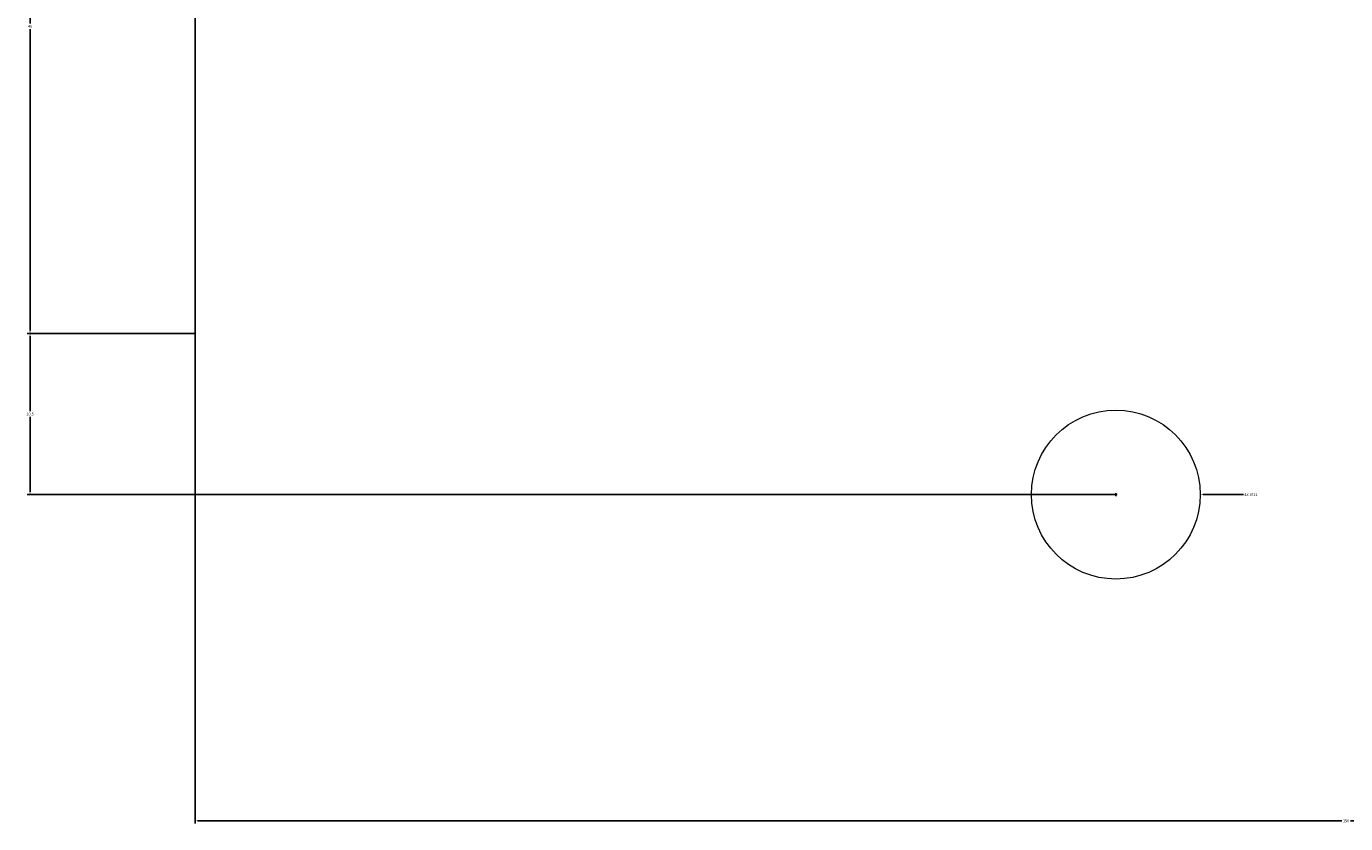
# Model space of a CAD drawing. Units: millimetres. Extents: x 315 to 487, y -72 to 32.
# Tile 1 of 4: x 315 to 401, y -72 to -20. Entities that reach past the tile are written whole.
import ezdxf

# ---------------------------------------------------------------- set-up
doc = ezdxf.new("R2010")
doc.units = ezdxf.units.MM
doc.layers.add('M-CONS', color=8, linetype='Continuous', lineweight=13)
doc.layers.add('M-DIMS', color=2, linetype='Continuous', lineweight=18)
doc.styles.get("Standard").update_dxf_attribs({"font": 'arial.ttf'})
doc.dimstyles.get("Standard").update_dxf_attribs({"dimtxt": 0.18, "dimasz": 0.18, "dimexe": 0.18, "dimexo": 0.0625, "dimgap": 0.09, "dimtad": 0, "dimtih": 1, "dimtoh": 1, "dimdec": 4, "dimzin": 0, "dimdsep": 46, "dimtxsty": 'Standard', "dimcen": 0.09, "dimadec": 0, "dimazin": 0, "dimtfac": 1, "dimtdec": 4, "dimtofl": 0, "dimtmove": 0, "dimatfit": 3, "dimfxl": 1, "dimtolj": 1, "dimtzin": 0, "dimarcsym": 0})

# ---------------------------------------------------------------- blocks, each defined once
blk = doc.blocks.new('*D3')
at = {"layer": 'Defpoints', "color": 0, "transparency": 16777216}
for p in [(326.007, 0), (476.007, 0), (476.007, -71.75)]:
    blk.add_point(p, dxfattribs=at)
at = {"layer": 'M-DIMS', "color": 0, "lineweight": -2, "transparency": 16777216}
for p, q in [((326.007, -0.062), (326.007, -71.93)), ((476.007, -0.062), (476.007, -71.93)), ((326.187, -71.75), (400.727, -71.75)), ((475.827, -71.75), (401.287, -71.75))]:
    blk.add_line(p, q, dxfattribs=at)
at = {"layer": 'M-DIMS', "color": 0, "transparency": 16777216}
for points in [[(326.187, -71.72), (326.187, -71.78), (326.007, -71.75)], [(475.827, -71.72), (475.827, -71.78), (476.007, -71.75)]]:
    blk.add_solid(points, dxfattribs=at)
at = {"layer": 'M-DIMS', "color": 0, "transparency": 16777216, "insert": (401.007, -71.75), "char_height": 0.18, "attachment_point": 5}
blk.add_mtext('\\A1;150', dxfattribs=at)
blk = doc.blocks.new('*D10')
at = {"layer": 'Defpoints', "color": 0, "transparency": 16777216}
for p in [(326.007, 0), (315.257, 0), (326.007, -40)]:
    blk.add_point(p, dxfattribs=at)
at = {"layer": 'M-DIMS', "color": 0, "lineweight": -2, "transparency": 16777216}
for p, q in [((325.945, 0), (315.077, 0)), ((315.257, -0.18), (315.257, -19.818)), ((315.257, -39.82), (315.257, -20.182)), ((325.945, -40), (315.077, -40))]:
    blk.add_line(p, q, dxfattribs=at)
at = {"layer": 'M-DIMS', "color": 0, "transparency": 16777216}
for points in [[(315.227, -0.18), (315.287, -0.18), (315.257, 0)], [(315.227, -39.82), (315.287, -39.82), (315.257, -40)]]:
    blk.add_solid(points, dxfattribs=at)
at = {"layer": 'M-DIMS', "color": 0, "transparency": 16777216, "insert": (315.257, -20), "char_height": 0.18, "attachment_point": 5}
blk.add_mtext('\\A1;40', dxfattribs=at)
blk = doc.blocks.new('*D13')
at = {"layer": 'Defpoints', "color": 0, "transparency": 16777216}
for p in [(315.257, -40), (326.007, -40), (386.007, -50.5)]:
    blk.add_point(p, dxfattribs=at)
at = {"layer": 'M-DIMS', "color": 0, "lineweight": -2, "transparency": 16777216}
for p, q in [((325.945, -40), (315.077, -40)), ((315.257, -40.18), (315.257, -45.068)), ((315.257, -50.32), (315.257, -45.432)), ((385.945, -50.5), (315.077, -50.5))]:
    blk.add_line(p, q, dxfattribs=at)
at = {"layer": 'M-DIMS', "color": 0, "transparency": 16777216}
for points in [[(315.227, -40.18), (315.287, -40.18), (315.257, -40)], [(315.227, -50.32), (315.287, -50.32), (315.257, -50.5)]]:
    blk.add_solid(points, dxfattribs=at)
at = {"layer": 'M-DIMS', "color": 0, "transparency": 16777216, "insert": (315.257, -45.25), "char_height": 0.18, "attachment_point": 5}
blk.add_mtext('\\A1;10.5', dxfattribs=at)
blk = doc.blocks.new('*D14')
at = {"layer": 'Defpoints', "color": 0, "transparency": 16777216}
for p in [(380.507, -50.5), (391.507, -50.5)]:
    blk.add_point(p, dxfattribs=at)
at = {"layer": 'M-DIMS', "color": 0, "lineweight": -2, "transparency": 16777216}
for p, q in [((385.917, -50.5), (386.097, -50.5)), ((386.007, -50.59), (386.007, -50.41)), ((394.316, -50.5), (391.687, -50.5))]:
    blk.add_line(p, q, dxfattribs=at)
at = {"layer": 'M-DIMS', "color": 0, "transparency": 16777216}
blk.add_solid([(391.687, -50.47), (391.687, -50.53), (391.507, -50.5)], dxfattribs=at)
at = {"layer": 'M-DIMS', "color": 0, "transparency": 16777216, "insert": (394.807, -50.5), "char_height": 0.18, "attachment_point": 5}
blk.add_mtext('\\A1;4X ∅11', dxfattribs=at)

msp = doc.modelspace()

# ---------------------------------------------------------------- linework, layer by layer
at = {"layer": 'M-CONS', "extrusion": (0, 1, 0)}
msp.add_line((326.007, 0, 200.054), (326.007, -40, 200.054), dxfattribs=at)
at = {"layer": 'M-CONS'}
msp.add_circle((386.007, -50.5, 200.054), 5.5, dxfattribs=at)

# ---------------------------------------------------------------- dimensions: what is measured, and where the dimension line sits
at = {"layer": 'M-DIMS'}
for base, p1, p2, override, picture, middle in [((315.257, 0), (326.007, -40), (326.007, 0), {"dimdec": 0, "dimlfac": 1, "dimrnd": 0, "dimzin": 0, "dimdsep": 46, "dimlunit": 2}, '*D10', (315.257, -20)), ((315.257, -40), (386.007, -50.5), (326.007, -40), {"dimdec": 1, "dimlfac": 1, "dimrnd": 0, "dimzin": 0, "dimdsep": 46, "dimlunit": 2}, '*D13', (315.257, -45.25))]:
    dim = msp.add_linear_dim(base=base, p1=p1, p2=p2, angle=90, dimstyle='Standard', override=override, dxfattribs=at)
    dim.commit()
    dim.dimension.update_dxf_attribs({"geometry": picture, "text_midpoint": middle})
dim = msp.add_linear_dim(base=(476.007, -71.75), p1=(326.007, 0), p2=(476.007, 0), dimstyle='Standard', override={"dimdec": 0, "dimlfac": 1, "dimrnd": 0, "dimzin": 0, "dimdsep": 46, "dimlunit": 2}, dxfattribs=at)
dim.commit()
dim.dimension.update_dxf_attribs({"geometry": '*D3', "text_midpoint": (401.007, -71.75)})
dim = msp.add_diameter_dim_2p(p1=(380.507, -50.5), p2=(391.507, -50.5), text='4X <>', dimstyle='Standard', override={"dimdec": 0, "dimlfac": 1, "dimrnd": 0, "dimzin": 0, "dimdsep": 46, "dimlunit": 2}, dxfattribs=at)
dim.commit()
dim.dimension.update_dxf_attribs({"geometry": '*D14', "text_midpoint": (394.807, -50.5), "dimtype": 163})

doc.saveas('drawing.dxf')
